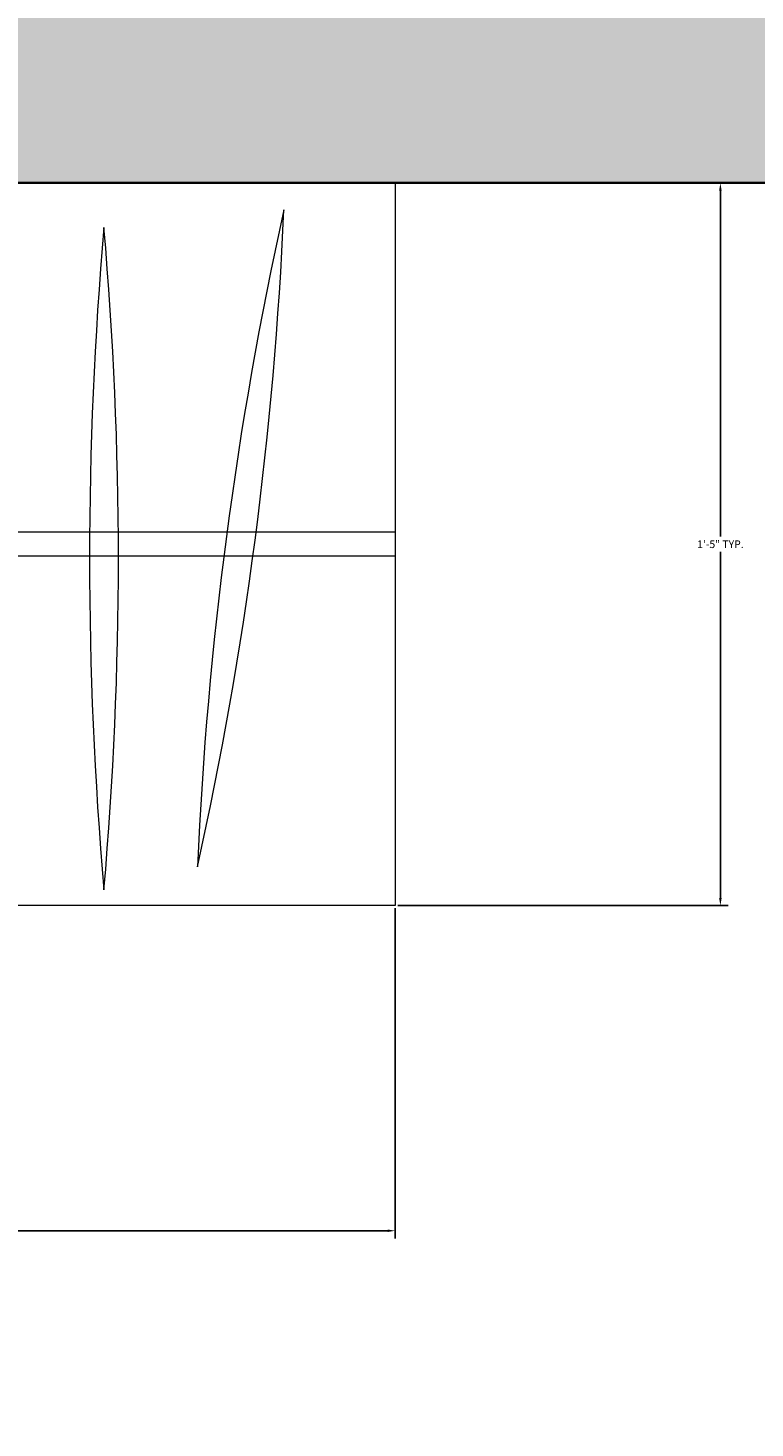
# Model space of a CAD drawing. Units: inches. Extents: x -9 to 505, y -680 to 48.
# Tile 11 of 17: x 79 to 96, y -198 to -165. Entities that reach past the tile are written whole.
import ezdxf

# ---------------------------------------------------------------- set-up
doc = ezdxf.new("R2010")
doc.units = ezdxf.units.IN
doc.header["$MEASUREMENT"] = 0
for name, color, linetype, lineweight in [('A-ANNO-DIMS', 2, 'Continuous', 18), ('A-FLOR-CASE', 8, 'Continuous', 18), ('A-WALL', 7, 'Continuous', 35), ('A-WALL-PATT', 251, 'Continuous', 13)]:
    doc.layers.add(name, color=color, linetype=linetype, lineweight=lineweight)
doc.styles.get("Standard").update_dxf_attribs({"font": 'arial.ttf'})
doc.dimstyles.get("Standard").update_dxf_attribs({"dimtxt": 0.18, "dimasz": 0.18, "dimexe": 0.18, "dimexo": 0.0625, "dimgap": 0.09, "dimtad": 0, "dimtih": 1, "dimtoh": 1, "dimdec": 0, "dimzin": 0, "dimdsep": 46, "dimlunit": 3, "dimtxsty": 'Standard', "dimcen": 0.09, "dimadec": 0, "dimazin": 0, "dimtfac": 1, "dimtdec": 0, "dimtofl": 0, "dimtmove": 0, "dimatfit": 3, "dimfxl": 1, "dimtolj": 1, "dimtzin": 0, "dimarcsym": 0})

# ---------------------------------------------------------------- blocks, each defined once
blk = doc.blocks.new('WARDROBE-HANGING')
for p, q in [((51.194, 17.065), (0, 17.065)), ((51.194, 17.065), (51.194, 0)), ((51.194, 8.817), (0, 8.817)), ((51.194, 8.248), (0, 8.248)), ((51.194, 0), (0, 0))]:
    blk.add_line(p, q)
for centre, start, end in [((136.229, -2.996), 167.50795, 177.50233), ((-41.142, 20.34), 347.50795, 357.50233), ((133.763, 8.192), 175.00281, 184.99719), ((-45.137, 8.192), 355.00281, 4.99719)]:
    blk.add_arc(centre, 89.791, start, end)
blk = doc.blocks.new('*D22')
at = {"layer": 'A-ANNO-DIMS', "color": 0, "lineweight": -2, "transparency": 16777216}
for p, q in [((36.264, -185.628), (36.264, -193.425)), ((87.458, -185.628), (87.458, -193.425)), ((36.444, -193.245), (60.443, -193.245)), ((87.278, -193.245), (63.279, -193.245))]:
    blk.add_line(p, q, dxfattribs=at)
at = {"layer": 'A-ANNO-DIMS', "color": 0, "transparency": 16777216}
for points in [[(36.444, -193.215), (36.444, -193.275), (36.264, -193.245)], [(87.278, -193.215), (87.278, -193.275), (87.458, -193.245)]]:
    blk.add_solid(points, dxfattribs=at)
at = {"layer": 'Defpoints', "color": 0, "transparency": 16777216}
for p in [(36.264, -185.566), (87.458, -185.566), (87.458, -193.245)]:
    blk.add_point(p, dxfattribs=at)
at = {"layer": 'A-ANNO-DIMS', "color": 0, "transparency": 16777216, "insert": (61.861, -193.245), "char_height": 0.18, "attachment_point": 5}
blk.add_mtext('\\A1;WARDROBE 4\'-3" TYP.', dxfattribs=at)
blk = doc.blocks.new('*D23')
at = {"layer": 'A-ANNO-DIMS', "color": 0, "lineweight": -2, "transparency": 16777216}
for p, q in [((87.521, -168.501), (95.318, -168.501)), ((95.138, -168.681), (95.138, -176.851)), ((95.138, -185.386), (95.138, -177.215)), ((87.521, -185.566), (95.318, -185.566))]:
    blk.add_line(p, q, dxfattribs=at)
at = {"layer": 'A-ANNO-DIMS', "color": 0, "transparency": 16777216}
for points in [[(95.108, -168.681), (95.168, -168.681), (95.138, -168.501)], [(95.108, -185.386), (95.168, -185.386), (95.138, -185.566)]]:
    blk.add_solid(points, dxfattribs=at)
at = {"layer": 'Defpoints', "color": 0, "transparency": 16777216}
for p in [(87.458, -168.501), (95.138, -168.501), (87.458, -185.566)]:
    blk.add_point(p, dxfattribs=at)
at = {"layer": 'A-ANNO-DIMS', "color": 0, "transparency": 16777216, "insert": (95.138, -177.033), "char_height": 0.18, "attachment_point": 5}
blk.add_mtext('\\A1;1\'-5" TYP.', dxfattribs=at)

msp = doc.modelspace()

# ---------------------------------------------------------------- hatches: boundary and pattern name
at = {"layer": 'A-WALL-PATT'}
h = msp.add_hatch(color=256, dxfattribs=at)
h.dxf.hatch_style = 1
h.paths.add_polyline_path([(101.641, 11.499), (48.264, 11.499), (48.264, 2.499), (72.264, 2.499), (72.264, -21.248), (81.264, -21.248), (81.264, 2.499), (101.641, 2.499)])
h.paths.add_polyline_path([(36.264, 2.499), (27.264, 2.499), (27.264, -6.918), (36.264, -6.918)])
h.paths.add_polyline_path([(81.264, -57.248), (72.264, -57.248), (72.264, -75.501), (81.264, -75.501)])
h.paths.add_polyline_path([(162.764, 11.499), (137.641, 11.499), (137.641, 2.499), (162.764, 2.499)])
h.paths.add_polyline_path([(179.264, 2.499), (174.764, 2.499), (174.764, -75.501), (179.264, -75.501), (179.264, -54.501), (229.514, -54.501), (229.514, -45.501), (179.264, -45.501)])
h.paths.add_polyline_path([(382.256, -45.501), (332.264, -45.501), (332.264, 2.499), (327.764, 2.499), (327.764, -45.501), (277.514, -45.501), (277.514, -54.501), (327.764, -54.501), (327.764, -111.501), (332.264, -111.501), (332.264, -54.501), (382.256, -54.501)])
h.paths.add_polyline_path([(332.264, -128.001), (327.764, -128.001), (327.764, -207.001), (332.264, -207.001)])
h.paths.add_polyline_path([(124.764, -111.501), (36.264, -111.501), (36.264, -116.001), (120.264, -116.001), (120.264, -168.501), (179.264, -168.501), (179.264, -164.001), (124.764, -164.001)])
h.paths.add_polyline_path([(96.264, -164.001), (36.264, -164.001), (36.264, -152.001), (27.264, -152.001), (27.264, -208.879), (36.264, -208.879), (36.264, -168.501), (96.264, -168.501)])
h.paths.add_polyline_path([(36.264, -244.879), (27.264, -244.879), (27.264, -287.001), (36.264, -287.001)])
h.paths.add_polyline_path([(179.264, -204.501), (174.764, -204.501), (174.764, -287.001), (179.264, -287.001)])
h.paths.add_polyline_path([(257.264, -296.001), (248.264, -296.001), (248.264, -446.001), (269.264, -446.001), (269.264, -437.001), (257.264, -437.001)])
h.paths.add_polyline_path([(90.264, -296.001), (81.264, -296.001), (81.264, -348.67), (90.264, -348.67)])
h.paths.add_polyline_path([(90.264, -384.67), (81.264, -384.67), (81.264, -416.001), (90.264, -416.001)])
h.paths.add_polyline_path([(170.264, -452.001), (36.264, -452.001), (36.264, -456.501), (165.764, -456.501), (165.764, -504.501), (165.133, -504.501), (165.133, -509.001), (170.264, -509.001)])
h.paths.add_polyline_path([(141.764, -504.501), (36.264, -504.501), (36.264, -492.501), (27.264, -492.501), (27.264, -565.959), (36.264, -565.959), (36.264, -509.001), (141.764, -509.001)])
h.paths.add_polyline_path([(36.264, -601.959), (27.264, -601.959), (27.264, -658.501), (36.264, -658.501)])
h.paths.add_polyline_path([(170.264, -670.501), (170.264, -634.501), (222.764, -634.501), (222.764, -625.501), (165.764, -625.501), (165.764, -670.501), (36.264, -670.501), (36.264, -679.501), (170.264, -679.501)])
h.paths.add_polyline_path([(332.264, -616.501), (433.894, -616.501), (433.894, -612.001), (332.264, -612.001), (332.264, -610.563), (327.764, -610.563), (327.764, -625.501), (270.764, -625.501), (270.764, -634.501), (327.764, -634.501), (327.764, -658.501), (332.264, -658.501)])
h.paths.add_polyline_path([(459.764, -670.501), (336.764, -670.501), (336.764, -679.501), (459.764, -679.501)])
h.paths.add_polyline_path([(468.764, -545.737), (459.764, -545.737), (459.764, -612.001), (457.894, -612.001), (457.894, -616.501), (459.764, -616.501), (459.764, -658.501), (468.764, -658.501)])
h.paths.add_polyline_path([(332.264, -446.001), (327.764, -446.001), (327.764, -574.563), (332.264, -574.563)])
h.paths.add_polyline_path([(327.764, -437.001), (305.264, -437.001), (305.264, -446.001), (327.764, -446.001)])
h.paths.add_polyline_path([(459.764, -437.001), (348.764, -437.001), (348.764, -446.001), (459.764, -446.001)])
h.paths.add_polyline_path([(468.764, -458.001), (459.764, -458.001), (459.764, -509.737), (468.764, -509.737)])
h.paths.add_polyline_path([(468.764, -365.001), (459.764, -365.001), (459.764, -437.001), (468.764, -437.001)])
h.paths.add_polyline_path([(468.764, -299.601), (459.764, -299.601), (459.764, -344.001), (468.764, -344.001)])
h.paths.add_polyline_path([(468.764, -184.739), (459.764, -184.739), (459.764, -231.001), (401.264, -231.001), (401.264, -235.501), (459.764, -235.501), (459.764, -275.601), (468.764, -275.601)])
h.paths.add_polyline_path([(390.764, -356.001), (342.764, -356.001), (342.764, -365.001), (390.764, -365.001)])
h.paths.add_polyline_path([(459.764, -356.001), (405.764, -356.001), (405.764, -365.001), (459.764, -365.001)])
h.paths.add_polyline_path([(405.764, -296.001), (396.764, -296.001), (396.764, -356.001), (405.764, -356.001)])
h.paths.add_polyline_path([(336.764, -296.001), (327.764, -296.001), (327.764, -356.001), (336.764, -356.001)])
h.paths.add_polyline_path([(468.764, -9.501), (459.764, -9.501), (459.764, -45.501), (418.256, -45.501), (418.256, -54.501), (468.764, -54.501)])
h.paths.add_polyline_path([(468.764, -54.501), (459.764, -54.501), (459.764, -111.501), (468.764, -111.501)])
h.paths.add_polyline_path([(468.764, -128.001), (459.764, -128.001), (459.764, -148.739), (468.764, -148.739)])

# ---------------------------------------------------------------- linework, layer by layer
at = {"layer": 'A-WALL'}
msp.add_line((36.264, -168.501), (179.264, -168.501), dxfattribs=at)

# ---------------------------------------------------------------- block references
at = {"layer": 'A-FLOR-CASE'}
msp.add_blockref('WARDROBE-HANGING', (36.264, -185.566), dxfattribs=at)

# ---------------------------------------------------------------- dimensions: what is measured, and where the dimension line sits
at = {"layer": 'A-ANNO-DIMS'}
dim = msp.add_linear_dim(base=(95.138, -168.501), p1=(87.458, -185.566), p2=(87.458, -168.501), angle=90, text='<> TYP.', dimstyle='Standard', override={"dimdec": 1, "dimlfac": 1, "dimrnd": 0, "dimzin": 1, "dimdsep": 46, "dimlunit": 4, "dimfrac": 2}, dxfattribs=at)
dim.commit()
dim.dimension.update_dxf_attribs({"geometry": '*D23', "text_midpoint": (95.138, -177.033)})
dim = msp.add_linear_dim(base=(87.458, -193.245), p1=(36.264, -185.566), p2=(87.458, -185.566), text='WARDROBE <> TYP.', dimstyle='Standard', override={"dimdec": 1, "dimlfac": 1, "dimrnd": 0, "dimzin": 1, "dimdsep": 46, "dimlunit": 4, "dimfrac": 2}, dxfattribs=at)
dim.commit()
dim.dimension.update_dxf_attribs({"geometry": '*D22', "text_midpoint": (61.861, -193.245)})

doc.saveas('drawing.dxf')
